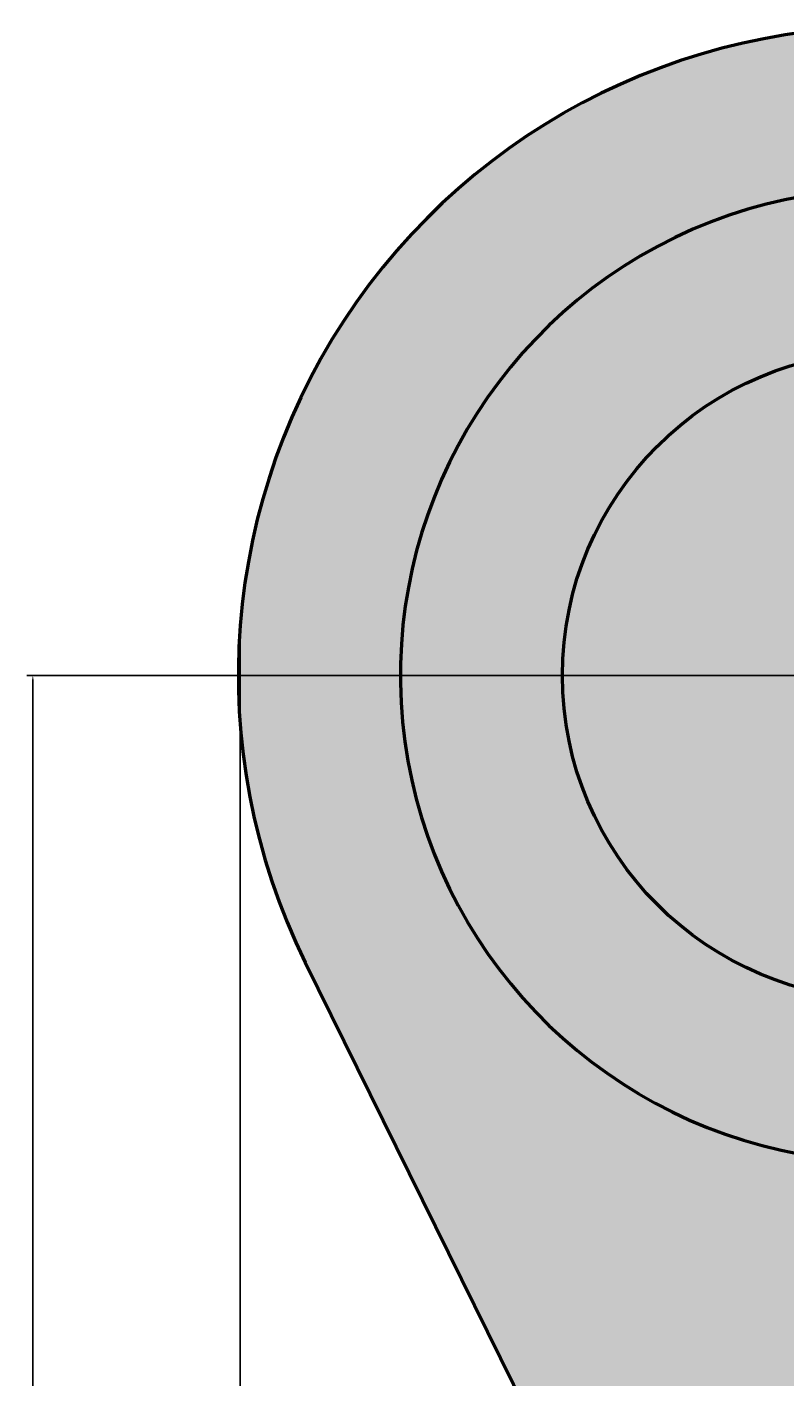
# Model space of a CAD drawing. Units: inches. Extents: x -31 to 87, y -18 to 100.
# Tile 3 of 7: x -31 to -8, y 52 to 93. Entities that reach past the tile are written whole.
import ezdxf

# ---------------------------------------------------------------- set-up
doc = ezdxf.new("R2010")
doc.units = ezdxf.units.IN
doc.header["$MEASUREMENT"] = 0
for name, color, linetype, lineweight in [('M-DIMS', 2, 'Continuous', 18), ('M-HATC', 7, 'Continuous', 18), ('M-OUTL', 4, 'Continuous', 50)]:
    doc.layers.add(name, color=color, linetype=linetype, lineweight=lineweight)
doc.styles.get("Standard").update_dxf_attribs({"font": 'arial.ttf'})
doc.dimstyles.get("Standard").update_dxf_attribs({"dimtxt": 0.18, "dimasz": 0.18, "dimexe": 0.18, "dimexo": 0.0625, "dimgap": 0.09, "dimtad": 0, "dimtih": 1, "dimtoh": 1, "dimdec": 4, "dimzin": 0, "dimdsep": 46, "dimtxsty": 'Standard', "dimcen": 0.09, "dimadec": 0, "dimazin": 0, "dimtfac": 1, "dimtdec": 4, "dimtofl": 0, "dimtmove": 0, "dimatfit": 3, "dimfxl": 1, "dimtolj": 1, "dimtzin": 0, "dimarcsym": 0})

# ---------------------------------------------------------------- blocks, each defined once
blk = doc.blocks.new('*D1')
at = {"layer": 'Defpoints', "color": 0, "transparency": 16777216}
for p in [(-24.622, 75.027), (80.28, 72.235), (80.28, -17.851)]:
    blk.add_point(p, dxfattribs=at)
at = {"layer": 'M-DIMS', "color": 0, "lineweight": -2, "transparency": 16777216}
for p, q in [((-24.622, 74.965), (-24.622, -18.031)), ((80.28, 72.173), (80.28, -18.031)), ((-24.442, -17.851), (27.443, -17.851)), ((80.1, -17.851), (28.214, -17.851))]:
    blk.add_line(p, q, dxfattribs=at)
at = {"layer": 'M-DIMS', "color": 0, "transparency": 16777216}
for points in [[(-24.442, -17.821), (-24.442, -17.881), (-24.622, -17.851)], [(80.1, -17.821), (80.1, -17.881), (80.28, -17.851)]]:
    blk.add_solid(points, dxfattribs=at)
at = {"layer": 'M-DIMS', "color": 0, "transparency": 16777216, "insert": (27.829, -17.851), "char_height": 0.18, "attachment_point": 5}
blk.add_mtext('\\A1;104.9', dxfattribs=at)
blk = doc.blocks.new('*D5')
at = {"layer": 'Defpoints', "color": 0, "transparency": 16777216}
for p in [(-31.022, 73.49), (-4.681, 73.49), (27.319, 8.49)]:
    blk.add_point(p, dxfattribs=at)
at = {"layer": 'M-DIMS', "color": 0, "lineweight": -2, "transparency": 16777216}
for p, q in [((-4.744, 73.49), (-31.202, 73.49)), ((-31.022, 73.31), (-31.022, 41.172)), ((-31.022, 8.67), (-31.022, 40.808)), ((27.256, 8.49), (-31.202, 8.49))]:
    blk.add_line(p, q, dxfattribs=at)
at = {"layer": 'M-DIMS', "color": 0, "transparency": 16777216}
for points in [[(-31.052, 73.31), (-30.992, 73.31), (-31.022, 73.49)], [(-31.052, 8.67), (-30.992, 8.67), (-31.022, 8.49)]]:
    blk.add_solid(points, dxfattribs=at)
at = {"layer": 'M-DIMS', "color": 0, "transparency": 16777216, "insert": (-31.022, 40.99), "char_height": 0.18, "attachment_point": 5}
blk.add_mtext('\\A1;65', dxfattribs=at)

msp = doc.modelspace()

# ---------------------------------------------------------------- hatches: boundary and pattern name
at = {"layer": 'M-HATC'}
h = msp.add_hatch(color=256, dxfattribs=at)
h.set_gradient(color1=(205, 32, 39), color2=(247, 242, 129))
h.paths.add_polyline_path([(-2.425, 93.362, 0.593504), (-22.614, 64.635), (8.64, 1.342, 0.746388), (46.874, 4.293), (79.436, 67.614, 0.505151), (60.278, 93.49)])
h.paths.add_polyline_path([(49.486, 83.865, -1.392259), (62.663, 58.674, 0.510547), (40.663, 15.341, -1.641082), (14.002, 15.393, 0.505248), (-7.332, 58.726, -1.377138), (6.152, 83.865, 0.426931)], flags=16)
h.paths.add_polyline_path([(5.319, 73.49, -1), (-14.681, 73.49, -1)], flags=0)
h.paths.add_polyline_path([(70.319, 73.49, -1), (50.319, 73.49, -1)], flags=0)
h.paths.add_polyline_path([(37.319, 8.49, -1), (17.319, 8.49, -1)], flags=0)
h.paths.add_polyline_path([(6.152, 83.865, 1.377138), (-7.332, 58.726, -0.505248), (14.002, 15.393, 1.641082), (40.663, 15.341, -0.510547), (62.663, 58.674, 1.392259), (49.486, 83.865, -0.426931)], flags=0)
h = msp.add_hatch(color=256, dxfattribs=at)
h.dxf.hatch_style = 1
h.paths.add_polyline_path([(5.319, 73.49, 1), (-14.681, 73.49, 1)])
h.paths.add_polyline_path([(50.319, 73.49, 1), (70.319, 73.49, 1)])
h.paths.add_polyline_path([(37.319, 8.49, 1), (17.319, 8.49, 1)])

# ---------------------------------------------------------------- linework, layer by layer
at = {"layer": 'M-OUTL'}
msp.add_line((8.64, 1.342), (-22.614, 64.635), dxfattribs=at)
msp.add_circle((-4.681, 73.49), 10, dxfattribs=at)
for radius, start, end in [(20, 83.5229, 206.2801), (15, 43.7617, 259.8216)]:
    msp.add_arc((-4.681, 73.49), radius, start, end, dxfattribs=at)

# ---------------------------------------------------------------- dimensions: what is measured, and where the dimension line sits
at = {"layer": 'M-DIMS'}
dim = msp.add_linear_dim(base=(80.28, -17.851), p1=(-24.622, 75.027), p2=(80.28, 72.235), dimstyle='Standard', override={"dimdec": 1, "dimlfac": 1, "dimrnd": 0, "dimzin": 0, "dimdsep": 46, "dimlunit": 2}, dxfattribs=at)
dim.commit()
dim.dimension.update_dxf_attribs({"geometry": '*D1', "text_midpoint": (27.829, -17.851)})
dim = msp.add_linear_dim(base=(-31.022, 73.49), p1=(27.319, 8.49), p2=(-4.681, 73.49), angle=90, dimstyle='Standard', override={"dimdec": 0, "dimlfac": 1, "dimrnd": 0, "dimzin": 0, "dimdsep": 46, "dimlunit": 2}, dxfattribs=at)
dim.commit()
dim.dimension.update_dxf_attribs({"geometry": '*D5', "text_midpoint": (-31.022, 40.99)})

doc.saveas('drawing.dxf')
